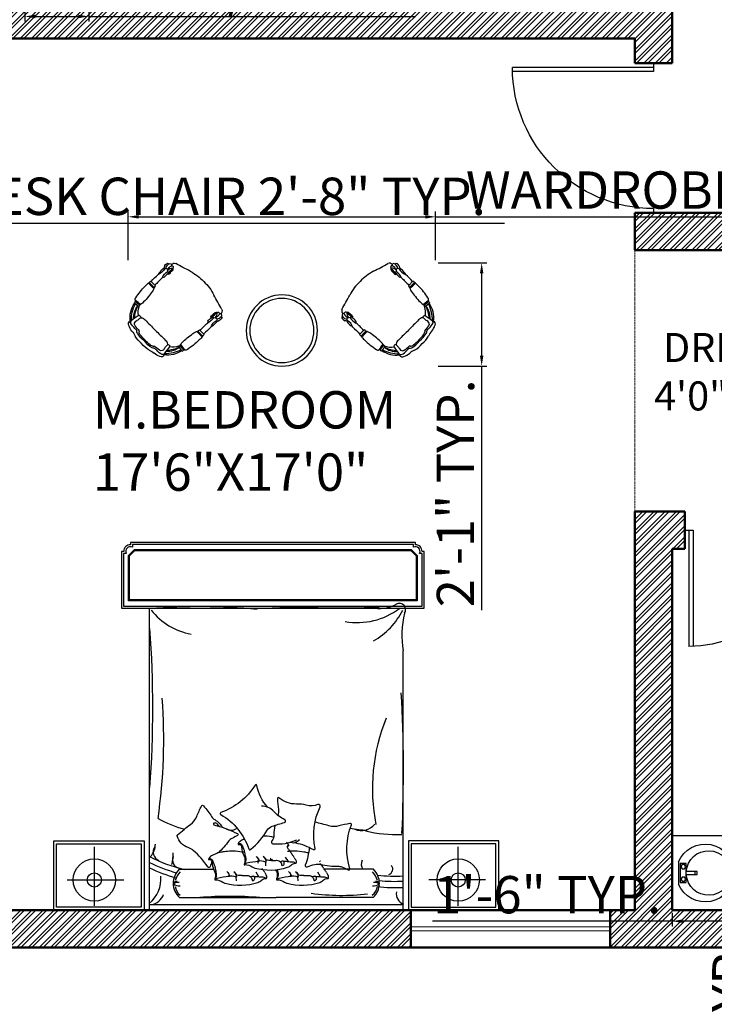
# Model space of a CAD drawing. Units: inches. Extents: x 3590 to 5167, y 65 to 1917.
# Tile 17 of 100: x 3716 to 3884, y 1312 to 1549. Entities that reach past the tile are written whole.
import ezdxf

# ---------------------------------------------------------------- set-up
doc = ezdxf.new("R2010")
doc.units = ezdxf.units.IN
doc.linetypes.add('DASHED', pattern=[0.75, 0.5, -0.25])
for name, color, linetype, lineweight in [('A-ANNO-DIMS', 2, 'Continuous', 18), ('A-AREA-IDEN', 7, 'Continuous', 18), ('A-DOOR', 3, 'Continuous', 25), ('A-FLOR-FIXT', 8, 'Continuous', 18), ('A-FURN', 21, 'Continuous', 18), ('A-GLAZ', 4, 'Continuous', 18), ('A-WALL', 7, 'Continuous', 50), ('A-WALL-PATT', 251, 'Continuous', 13), ('S-BEAM-OVHD', 7, 'DASHED', 18)]:
    doc.layers.add(name, color=color, linetype=linetype, lineweight=lineweight)
for name, color, linetype in [('FUR', 42, 'Continuous'), ('furn', 7, 'Continuous'), ('HA-FUR', 8, 'Continuous'), ('HA-P', 8, 'Continuous'), ('SAN', 5, 'Continuous'), ('SANTEH', 7, 'Continuous'), ('wood', 26, 'Continuous')]:
    doc.layers.add(name, color=color, linetype=linetype)
doc.styles.get("Standard").update_dxf_attribs({"font": 'arial.ttf'})
doc.dimstyles.new('ISO-25', dxfattribs={"dimtxt": 9, "dimasz": 2.5, "dimexe": 1.25, "dimexo": 0.625, "dimtad": 1, "dimdec": 1, "dimlunit": 3, "dimtxsty": 'Standard', "dimcen": 2.5, "dimadec": 0, "dimazin": 0, "dimtfac": 1, "dimtdec": 1, "dimtmove": 0, "dimatfit": 3, "dimfxl": 1, "dimarcsym": 0})

# ---------------------------------------------------------------- blocks, each defined once
blk = doc.blocks.new('D2')
for p, q in [((1, 0), (1, 28)), ((2, 0), (2, 27.98)), ((0, 0), (2, 0)), ((29, 0), (30, 0))]:
    blk.add_line(p, q)
at = {"ltscale": 0.5}
blk.add_arc((1, 0), 28, 0, 90, dxfattribs=at)
blk = doc.blocks.new('D1')
for p, q in [((1, 0), (1, 34)), ((2, 0), (2, 33.99)), ((0, 0), (2, 0)), ((35, 0), (36, 0))]:
    blk.add_line(p, q)
at = {"ltscale": 0.5}
blk.add_arc((1, 0), 34, 0, 90, dxfattribs=at)
blk = doc.blocks.new('r11')
at = {"layer": 'SANTEH', "ltscale": 5}
for p, q in [((0, 0), (600, 0)), ((0, -600), (0, 0)), ((600, 0), (600, -600)), ((210.5, -50), (389.5, -50)), ((210.5, -50), (210.5, -50)), ((223.8, -63.2), (376.2, -63.2)), ((223.8, -113.2), (223.8, -63.2)), ((232.7, -78.7), (249.2, -69.1)), ((232.7, -97.7), (232.7, -78.7)), ((249.2, -69.1), (265.7, -78.7)), ((265.7, -78.7), (265.7, -97.7)), ((334.3, -78.7), (350.8, -69.1)), ((334.3, -97.7), (334.3, -78.7)), ((350.8, -69.1), (367.3, -78.7)), ((367.3, -78.7), (367.3, -97.7)), ((376.2, -63.2), (376.2, -113.2)), ((376.2, -113.2), (223.8, -113.2)), ((249.2, -107.2), (232.7, -97.7)), ((265.7, -97.7), (249.2, -107.2)), ((288, -201.6), (288, -113.2)), ((312, -113.2), (312, -201.6)), ((350.8, -107.2), (334.3, -97.7)), ((367.3, -97.7), (350.8, -107.2)), ((312, -184.3), (288, -184.3)), ((312, -201.6), (288, -201.6)), ((600, -600), (0, -600))]:
    blk.add_line(p, q, dxfattribs=at)
for centre, radius, start, end in [((300, -266.2), 234, 112.50001, 67.49999), ((300, -293), 180.2, 93.8183, 86.1817)]:
    blk.add_arc(centre, radius, start, end, dxfattribs=at)
blk = doc.blocks.new('A$C0A42580C')
at = {"layer": 'SAN'}
for p, q in [((0.2873, 0.0301), (0.2873, 0.4484)), ((2.8678, 0.0301), (2.8678, 0.4484)), ((0.0949, 0.2135), (0.4958, 0.2135)), ((3.0601, 0.2135), (2.6592, 0.2135))]:
    blk.add_line(p, q, dxfattribs=at)
for centre, radius in [((0.2873, 0.2135), 0.15), ((2.8678, 0.2135), 0.15), ((0.2873, 0.2135), 0.05), ((2.8678, 0.2135), 0.05)]:
    blk.add_circle(centre, radius, dxfattribs=at)
at = {"layer": 'wood'}
for p, q in [((0.6775, 0.8851), (0.6775, 2.1392)), ((2.4775, 0.8016), (2.4775, 1.838)), ((2.4775, 0), (2.4775, 0.8016)), ((1.6633, 0.3438), (1.6434, 0.3761)), ((0.888, 0.289), (1.1327, 0.289)), ((1.5, 0.3423), (1.5016, 0.3142)), ((2.267, 0.289), (1.9163, 0.289)), ((1.2906, 0.2348), (1.2921, 0.2067)), ((1.4538, 0.2362), (1.434, 0.2685)), ((1.7287, 0.2348), (1.7302, 0.2067)), ((1.8919, 0.2362), (1.8721, 0.2685)), ((0.8909, 0.089), (1.5775, 0.089)), ((2.2642, 0.089), (1.5775, 0.089)), ((0.6775, 0.039), (2.4775, 0.039)), ((0.6775, 0), (2.4775, 0))]:
    blk.add_line(p, q, dxfattribs=at)
blk.add_lwpolyline([(0.6775, 0), (0.6775, 0.8851)], dxfattribs=at)
for points in [[(1.516, 0.7294, -0.128392), (1.4401, 0.8834, 0.70791), (1.427, 0.8863, -0.16964), (1.1848, 0.6919, 0.664036), (1.184, 0.6776, -0.184649), (1.3819, 0.4332, 0.662242), (1.3969, 0.4309, 0.078539), (1.5137, 0.5669, -0.1736), (1.5484, 0.5947, -0.02159), (1.6357, 0.6205, 0.697276), (1.6379, 0.6405, -0.093019), (1.5606, 0.699, 0.216632), (1.4719, 0.7371, -2.511293)], [(1.6795, 0.4818, 0.263265), (1.7191, 0.4839, -0.026108), (1.743, 0.4973, 0.027613), (1.7137, 0.4764, -0.089259), (1.8403, 0.429, 0.662242), (1.8528, 0.4376, -0.162037), (1.8882, 0.732, 0.676499), (1.8733, 0.748, -0.160513), (1.7901, 0.7439, 0.07473), (1.7202, 0.7523, -0.187721), (1.5966, 0.7963, 0.70791), (1.5851, 0.7895, -0.010003), (1.5921, 0.7143, -0.07079), (1.5891, 0.6719, 0.099539)], [(1.1211, 0.3454, 0.032543), (1.1095, 0.3091, -0.658965), (1.0917, 0.3063, 0.074753), (0.9887, 0.4234, 0.100988), (0.953, 0.4429, -0.270711), (0.8753, 0.5273, -0.276825), (0.8775, 0.5337, -0.014937), (0.9701, 0.6081, 0.134834), (1.0135, 0.6643, -0.023706), (1.0474, 0.7372, -0.664036), (1.0616, 0.7394, -0.035987), (1.119, 0.6627, 0.118631), (1.1415, 0.6412, -0.132738), (1.1955, 0.5864)], [(1.1759, 0.5928, 0.013884), (1.1549, 0.6131, 0.174178), (1.1437, 0.6177, 0.104076), (1.1358, 0.6165, 0.389829), (1.1324, 0.6097, 0.296089), (1.1415, 0.6019, -0.036701), (1.1572, 0.5985, -0.040547), (1.3022, 0.543, -0.70791), (1.3021, 0.5296, -0.016811), (1.2631, 0.5085, 0.11866), (1.2414, 0.4904, -0.048791), (1.1649, 0.4055, 0.103757)], [(1.5674, 0.601, 0.057807), (1.5606, 0.5339, -0.173425), (1.5457, 0.49, 0.589988), (1.5538, 0.4706, 0.137312), (1.7236, 0.4985, 0.137312)], [(1.8113, 0.4446, -0.069098), (1.7831, 0.3187, 0.658965), (1.7961, 0.3062, -0.049789), (1.8516, 0.3234, -0.103757), (1.8905, 0.3233, 0.055725), (2.0203, 0.3103, -0.11866), (2.0478, 0.304, 0.016811), (2.0881, 0.2856, 0.70791), (2.0989, 0.2936, -0.16964), (2.1104, 0.604, 0.664036), (2.1001, 0.6139, 0.023706), (2.0214, 0.597, -0.134834), (1.9505, 0.5976, 0.012748), (1.8522, 0.6228)], [(1.3107, 0.4764, 0.145733), (1.3069, 0.4677, 0.488583), (1.3089, 0.4657, -0.012138), (1.3131, 0.4661, -0.125673), (1.3213, 0.4646, -0.750706)], [(1.3153, 0.4751, -0.274893), (1.3379, 0.4529, 0.051436), (1.3468, 0.4293, -0.086628), (1.3532, 0.4078, 0.040196), (1.3593, 0.3772, -0.184744), (1.3556, 0.3344, -2.554464)], [(1.317, 0.4683, -0.060098), (1.3283, 0.4571, -0.16247), (1.3313, 0.4487, 0.120018), (1.3493, 0.3815, -0.060072), (1.3541, 0.3695, -0.13107), (1.3541, 0.3395, -0.024415), (1.3534, 0.3373, 0.070398), (1.3503, 0.3233, 0.528689), (1.3524, 0.3216, -0.069388), (1.3557, 0.3222, -0.158233), (1.4075, 0.3065, 0.085461), (1.4255, 0.2981, 0.147196), (1.6571, 0.3041, 0.10985), (1.6823, 0.3191, -0.179095), (1.7126, 0.3319, -2.318897)], [(1.1013, 0.3688, 0.145733), (1.0975, 0.3601, 0.488583), (1.0995, 0.3581, -0.012138), (1.1036, 0.3585, -0.125673), (1.1119, 0.357, -0.750706)], [(1.1059, 0.3675, -0.274893), (1.1285, 0.3453, 0.051436), (1.1373, 0.3217, -0.086628), (1.1438, 0.3003, 0.040196), (1.1499, 0.2696, -0.184744), (1.1462, 0.2269, -2.554464)], [(1.1076, 0.3607, -0.060098), (1.1189, 0.3495, -0.16247), (1.1219, 0.3411, 0.120018), (1.1399, 0.2739, -0.060072), (1.1447, 0.2619, -0.13107), (1.1447, 0.2319, -0.024415), (1.144, 0.2297, 0.070398), (1.1409, 0.2157, 0.528689), (1.143, 0.2141, -0.069388), (1.1463, 0.2146, -0.158233), (1.1981, 0.1989, 0.085461), (1.2161, 0.1905, 0.147196), (1.4477, 0.1965, 0.10985), (1.4728, 0.2115, -0.179095), (1.5032, 0.2244, -2.318897)], [(1.4359, 0.3803, -0.198519), (1.452, 0.3494, 0.826402), (1.4558, 0.349, 0.095956), (1.4561, 0.3528, 0.242899), (1.4461, 0.3686, -17.523452)], [(1.5447, 0.3525, -0.083557), (1.507, 0.3546, 0.203162), (1.4851, 0.3792, -0.208037), (1.5043, 0.3409, 0.124669), (1.4432, 0.3469, 0.965934)], [(1.5394, 0.3688, 0.145733), (1.5356, 0.3601, 0.488583), (1.5376, 0.3581, -0.012138), (1.5418, 0.3585, -0.125673), (1.55, 0.357, -0.750706)], [(1.5447, 0.3525, -0.008229), (1.5728, 0.3519, 0.033691)], [(1.5728, 0.3519, -0.46905), (1.6152, 0.321, 0.420988), (1.62, 0.3169, 0.857652), (1.6221, 0.3484, 0.548526)], [(1.3509, 0.3219, -0.117141), (1.3688, 0.335, -0.025084), (1.4533, 0.348, 0.033691)], [(1.5721, 0.286, 0.022869), (1.578, 0.2739, -0.060072), (1.5828, 0.2619, -0.13107), (1.5828, 0.2319, -0.024415), (1.5821, 0.2297, 0.070398), (1.579, 0.2157, 0.528689), (1.5811, 0.2141, -0.069388), (1.5844, 0.2146, -0.158233), (1.6362, 0.1989, 0.085461), (1.6542, 0.1905, 0.147196), (1.8858, 0.1965, 0.10985), (1.911, 0.2115, -0.179095), (1.9413, 0.2244, -2.318897)], [(1.5838, 0.2873, 0.023398), (1.588, 0.2696, -0.184744), (1.5843, 0.2269, -2.554464)], [(1.603, 0.3451, -0.099719), (1.6221, 0.3484, 0.102691)], [(1.6214, 0.3487, -0.010168), (1.6558, 0.3447, 0.033691), (1.6907, 0.3423, -0.220869), (1.7148, 0.3311, -0.288972)], [(1.1415, 0.2143, -0.117141), (1.1594, 0.2274, -0.025084), (1.2439, 0.2405, 0.033691)], [(1.2265, 0.2728, -0.198519), (1.2426, 0.2418, 0.826402), (1.2463, 0.2415, 0.095956), (1.2467, 0.2452, 0.242899), (1.2366, 0.2611, -17.523452)], [(1.3353, 0.2449, -0.083557), (1.2976, 0.247, 0.203162), (1.2757, 0.2717, -0.208037), (1.2948, 0.2333, 0.124669), (1.2338, 0.2393, 0.965934)], [(1.3353, 0.2449, -0.008229), (1.3633, 0.2443, 0.033691)], [(1.3633, 0.2443, -0.46905), (1.4058, 0.2134, 0.420988), (1.4106, 0.2093, 0.857652), (1.4127, 0.2408, 0.548526)], [(1.3936, 0.2375, -0.099719), (1.4127, 0.2408, 0.102691)], [(1.412, 0.2411, -0.010168), (1.4464, 0.2371, 0.033691), (1.4812, 0.2348, -0.220869), (1.5054, 0.2235, -0.288972)], [(1.5796, 0.2143, -0.117141), (1.5975, 0.2274, -0.025084), (1.682, 0.2405, 0.033691)], [(1.6646, 0.2728, -0.198519), (1.6807, 0.2418, 0.826402), (1.6845, 0.2415, 0.095956), (1.6848, 0.2452, 0.242899), (1.6748, 0.2611, -17.523452)], [(1.7734, 0.2449, -0.083557), (1.7357, 0.247, 0.203162), (1.7138, 0.2717, -0.208037), (1.733, 0.2333, 0.124669), (1.6719, 0.2393, 0.965934)], [(1.7734, 0.2449, -0.008229), (1.8015, 0.2443, 0.033691)], [(1.8015, 0.2443, -0.46905), (1.8439, 0.2134, 0.420988), (1.8487, 0.2093, 0.857652), (1.8508, 0.2408, 0.548526)], [(1.8317, 0.2375, -0.099719), (1.8508, 0.2408, 0.102691)], [(1.8501, 0.2411, -0.010168), (1.8845, 0.2371, 0.033691), (1.9193, 0.2348, -0.220869), (1.9435, 0.2235, -0.288972)]]:
    blk.add_lwpolyline(points, format="xyb", dxfattribs=at)
for points in [[(0.64, 0), (0, 0), (0, 0.49), (0.64, 0.49)], [(2.515, 0), (3.155, 0), (3.155, 0.49), (2.515, 0.49)], [(0.62, 0.02), (0.02, 0.02), (0.02, 0.47), (0.62, 0.47)], [(2.535, 0.02), (3.135, 0.02), (3.135, 0.47), (2.535, 0.47)]]:
    blk.add_lwpolyline(points, close=True, dxfattribs=at)
for centre, radius, start, end in [((2.3125, 2.3833), 0.2443, 254.1515, 300.95574), ((2.4501, 2.1309), 0.0445, 324.18954, 118.92203), ((1.0344, -2.14), 4.292, 84.56078, 94.7164), ((1.0494, 2.4026), 0.4515, 217.47941, 260.35986), ((2.0208, -11.0786), 13.2288, 88.75549, 92.51133), ((2.1491, 2.5471), 0.5083, 260.65485, 306.44155), ((2.0168, 2.3573), 0.5127, 299.08175, 333.44367), ((3.1371, 1.9502), 0.669, 166.6404, 189.65708), ((-7.0839, 1.4328), 7.7858, 355.84817, 4.15183), ((-7.2439, 0.9937), 9.7233, 357.34474, 3.23068), ((-3.167, 1.2143), 3.9465, 351.77286, 4.18386), ((3.5803, 0.8622), 1.3213, 157.81295, 191.15154), ((1.1611, 1.4181), 0.8768, 241.21362, 254.41879), ((1.2583, 0.6364), 0.0695, 238.58923, 301.92671), ((1.7861, -2.1601), 2.7557, 80.89877, 83.46656), ((2.181, 0.6859), 0.1221, 247.37754, 321.13165), ((2.4192, 1.3819), 0.8461, 255.77539, 273.25587), ((1.3546, 0.4469), 0.0529, 114.21284, 146.15395), ((2.6126, -2.3504), 3.1201, 113.83178, 114.21284), ((1.4714, 0.0722), 0.4528, 80.62397, 88.74059), ((1.4035, -0.3388), 0.8693, 79.71489, 80.62397), ((0.5904, 0.4689), 0.13, 317.38218, 359.70393), ((0.7723, 0.4131), 0.0674, 147.68233, 245.79865), ((1.6301, 0.4539), 0.0342, 31.14095, 54.95422), ((1.6709, 0.4489), 0.0156, 131.9623, 212.08127), ((1.6729, 0.4422), 0.0178, 140.41793, 157.63267), ((1.7235, 0.4818), 0.0777, 212.08127, 227.364), ((1.6635, 0.4499), 0.00568, 95.52245, 140.41793), ((1.5664, 0.4154), 0.1086, 24.20989, 31.14095), ((1.6627, 0.4587), 0.00309, 275.52245, 24.20989), ((1.6391, 0.3902), 0.0469, 17.32618, 47.364), ((1.1611, 1.3191), 1.0568, 242.76671, 257.10398), ((0.0312, 0.4583), 0.8174, 350.42368, 356.2506), ((0.9021, 0.3562), 0.0605, 155.8342, 254.41058), ((1.1452, 0.3394), 0.0529, 114.21284, 146.15395), ((2.4032, -2.458), 3.1201, 113.55686, 114.21284), ((1.2046, 0.2912), 0.121, 99.42032, 113.55686), ((1.2774, -0.1478), 0.5659, 95.90379, 99.42032), ((1.2626, -0.005), 0.4223, 88.74059, 95.90379), ((1.2619, -0.0354), 0.4528, 80.62397, 88.74059), ((1.1941, -0.4464), 0.8693, 79.45871, 80.62397), ((1.4207, 0.3463), 0.0342, 31.14095, 54.95422), ((1.4614, 0.3413), 0.0156, 131.9623, 212.08127), ((1.357, 0.3078), 0.1086, 24.20989, 31.14095), ((1.4533, 0.3511), 0.00309, 275.52245, 24.20989), ((1.7007, -0.005), 0.4223, 88.74059, 95.90379), ((1.7106, 0.4125), 0.028, 197.32618, 226.17302), ((1.6431, 0.3422), 0.0695, 26.61764, 46.17302), ((1.8202, 0.431), 0.1287, 206.61764, 215.96192), ((1.7001, -0.0354), 0.4528, 80.62397, 88.74059), ((1.6975, 0.3419), 0.023, 350.76434, 35.96192), ((1.6322, -0.4464), 0.8693, 78.43923, 80.62397), ((2.2511, 0.3256), 0.071, 155.86842, 211.04513), ((1.1611, 1.3191), 1.0937, 243.75553, 254.4906), ((1.1611, 1.2816), 1.0937, 243.75553, 254.38927), ((0.9846, 0.1903), 0.1381, 134.39284, 227.23745), ((1.4635, 0.3347), 0.0178, 140.41793, 157.63267), ((1.4541, 0.3424), 0.00568, 95.52245, 140.41793), ((1.5012, 0.305), 0.028, 197.32618, 226.17302), ((1.4337, 0.2347), 0.0695, 26.61764, 46.17302), ((1.715, 0.3349), 0.00379, 207.1817, 328.02977), ((1.7058, 0.3406), 0.0145, 328.02977, 350.76434), ((1.9016, 0.3347), 0.0178, 140.41793, 157.63267), ((1.9522, 0.3743), 0.0777, 212.08127, 227.364), ((1.8922, 0.3424), 0.00568, 95.52245, 140.41793), ((1.8678, 0.2827), 0.0469, 17.32618, 47.364), ((1.9393, 0.305), 0.028, 197.32618, 226.17302), ((1.8718, 0.2347), 0.0695, 26.61764, 46.17302), ((2.1704, 0.1903), 0.1381, 312.76255, 45.60716), ((2.3616, 0.2915), 0.0419, 290.78583, 35.36309), ((0.5293, 0.2241), 0.2307, 309.63048, 4.27465), ((0.9986, 0.1735), 0.1427, 136.58239, 164.9725), ((1.6108, 0.3235), 0.1287, 206.61764, 215.96192), ((1.5055, 0.2273), 0.00379, 207.1817, 328.02977), ((1.4881, 0.2344), 0.023, 350.76434, 35.96192), ((1.4964, 0.233), 0.0145, 328.02977, 350.76434), ((2.0489, 0.3235), 0.1287, 206.61764, 215.96192), ((1.9436, 0.2273), 0.00379, 207.1817, 328.02977), ((1.9262, 0.2344), 0.023, 350.76434, 35.96192), ((1.9345, 0.233), 0.0145, 328.02977, 350.76434), ((2.1565, 0.1735), 0.1427, 15.0275, 43.41761), ((2.4192, 1.2667), 1.0261, 263.09035, 273.25587), ((2.4192, 1.2667), 1.0629, 263.94374, 273.25587), ((0.8396, 0.185), 0.0112, 314.89662, 45.10338), ((0.8413, 0.1846), 0.0128, 299.47062, 57.44416), ((0.8844, 0.2286), 0.0569, 229.70587, 281.11527), ((0.8802, 0.1371), 0.0592, 81.47786, 123.11925), ((0.8698, 0.1793), 0.0229, 77.14902, 159.1786), ((0.9466, 0.1765), 0.0862, 185.53723, 234.68694), ((2.2085, 0.1765), 0.0862, 305.31306, 354.46277), ((2.2706, 0.2286), 0.0569, 258.88473, 310.29413), ((2.2749, 0.1371), 0.0592, 56.88075, 98.52214), ((2.2853, 0.1793), 0.0229, 20.8214, 102.85098), ((2.4192, 1.2218), 1.0629, 263.23622, 273.25587), ((2.3138, 0.1846), 0.0128, 122.55584, 240.52938), ((2.3154, 0.185), 0.0112, 134.89662, 225.10338), ((0.6729, 0.151), 0.1135, 279.23824, 338.73819), ((1.2481, -2.5919), 2.6893, 85.4722, 94.5278), ((2.0447, 1.7022), 1.5979, 262.13639, 276.48786), ((2.508, 0.1152), 0.0792, 169.94668, 248.24015)]:
    blk.add_arc(centre, radius, start, end, dxfattribs=at)
blk = doc.blocks.new('A$C623F1DA0')
at = {"layer": 'FUR'}
blk.add_lwpolyline([(0.628, 2.912, 0.414214), (0.562, 2.978), (0.562, 3), (0, 3), (0, 0), (0.562, 0), (0.562, 0.022, 0.414214), (0.628, 0.088), (0.65, 0.088), (0.65, 2.912)], format="xyb", close=True, dxfattribs=at)
at = {"layer": 'HA-FUR'}
blk.add_lwpolyline([(0.6034, 2.892, 0.710288), (0.542, 2.9534), (0.542, 2.98), (0.02, 2.98), (0.02, 0.02), (0.542, 0.02), (0.542, 0.0466, 0.710288), (0.6034, 0.108), (0.63, 0.108), (0.63, 2.892)], format="xyb", close=True, dxfattribs=at)
at = {"layer": 'HA-P'}
for points in [[(0.07, 2.93), (0.5213, 2.93), (0.58, 2.8713), (0.58, 0.1287), (0.5213, 0.07), (0.07, 0.07)], [(0.08, 2.92), (0.5171, 2.92), (0.57, 2.8671), (0.57, 0.1329), (0.5171, 0.08), (0.08, 0.08)]]:
    blk.add_lwpolyline(points, close=True, dxfattribs=at)
blk = doc.blocks.new('CHAIR6')
at = {"layer": 'furn'}
for p, q in [((0.41, 0.26), (0.4094, 0.3185)), ((0.4281, 0.3181), (0.4272, 0.263)), ((0.41, -0.26), (0.4094, -0.3185)), ((0.4281, -0.3181), (0.4272, -0.263))]:
    blk.add_line(p, q, dxfattribs=at)
for centre in [(0.2174, 0.2867), (0.2187, 0.2766), (0.22, 0.2683), (0.2209, 0.2599), (0.2221, 0.2517), (0.4052, 0.3065), (0.4053, 0.3148), (0.4053, 0.2897), (0.4054, 0.2981), (0.4054, 0.2729), (0.4055, 0.2812), (0.4056, 0.2643), (0.2231, 0.2433), (0.2221, -0.2517), (0.2231, -0.2433), (0.2174, -0.2867), (0.2187, -0.2766), (0.22, -0.2683), (0.2209, -0.2599), (0.4052, -0.3065), (0.4053, -0.2897), (0.4053, -0.3148), (0.4054, -0.2981), (0.4054, -0.2729), (0.4055, -0.2812), (0.4056, -0.2643)]:
    blk.add_circle(centre, 0.00425, dxfattribs=at)
for centre, radius, start, end in [((0.2315, 0.0781), 0.2058, 99.53594, 142.96968), ((0.288, -0.009), 0.2959, 107.467, 135.69066), ((0.1998, 0.3299), 0.0425, 267.37882, 299.53851), ((0.5076, 0.3087), 0.3105, 183.92135, 193.66405), ((0.91, 0.35), 0.6998, 184.95819, 189.17441), ((0.2369, 0.2913), 0.0162, 83.97727, 174.0092), ((2.2364, 0.5463), 2.0315, 187.16408, 188.67417), ((0.3719, -0.3167), 0.6382, 90.6066, 102.05541), ((0.3772, 0.1685), 0.1534, 77.89638, 94.52684), ((0.357, 0.3514), 0.1057, 274.42127, 300.14813), ((3.3638, 0.3149), 2.9628, 179.90105, 181.14792), ((0.4178, 0.2794), 0.04, 75.21702, 102.18253), ((0.4118, 0.3013), 0.0413, 267.60688, 291.9537), ((0.4709, 1.0442), 0.7753, 266.77935, 273.30843), ((0.4807, -0.3094), 0.6241, 87.1388, 94.84242), ((0.5163, 0.348), 0.0344, 262.5365, 295.12391), ((0.5543, 0.4048), 0.1004, 244.96152, 286.92621), ((0.5583, 0.1491), 0.1284, 78.32163, 109.43704), ((0.5171, 0.2599), 0.0105, 7.92951, 98.404), ((0.5475, 0.4175), 0.1574, 262.69111, 279.4279), ((0.5573, 0.1986), 0.1211, 80.56871, 102.58021), ((0.5763, 0.2592), 0.00554, 151.0446, 320.63906), ((0.5726, 0.2536), 0.00119, 58.88827, 217.83169), ((0.5864, 0.2986), 0.0481, 252.15364, 277.04405), ((0.5749, 0.272), 0.00992, 261.06044, 17.03518), ((0.569, 0.3057), 0.0148, 11.93121, 56.71364), ((0.6, 0.6108), 0.3491, 266.32513, 275.76594), ((0.5857, 0.2587), 0.00592, 143.235, 315.8485), ((0.5574, 0.3682), 0.0592, 293.70731, 312.31146), ((0.5811, 0.2921), 0.0168, 1.95853, 81.75781), ((0.5706, 0.2994), 0.0282, 299.26311, 346.05528), ((0.54, 0.2614), 0.0504, 352.19447, 0.49312), ((0.5958, 0.265), 0.012, 240.91565, 292.3604), ((0.5993, 0.2232), 0.0286, 84.23587, 104.22566), ((0.6205, 0.2416), 0.0492, 62.08685, 124.06689), ((0.5958, 0.2324), 0.05, 38.36456, 93.27362), ((0.6272, 0.2528), 0.0606, 83.33143, 123.59051), ((0.6147, 0.2731), 0.0542, 72.72663, 108.72189), ((0.6298, 0.2592), 0.03, 175.25421, 190.14236), ((0.6039, 0.2608), 0.00773, 242.68072, 299.22641), ((0.6055, 0.322), 0.0704, 267.27867, 279.33441), ((0.6233, 0.2599), 0.0167, 173.50236, 200.39748), ((0.6103, 0.2582), 0.0049, 236.84733, 330.71615), ((0.6462, 0.2619), 0.0322, 179.91617, 191.03659), ((0.6177, 0.2574), 0.00347, 207.27606, 12.12043), ((0.6201, 0.2638), 0.0117, 254.38571, 324.07897), ((0.7103, 0.267), 0.0896, 182.99093, 185.70819), ((0.6264, 0.2651), 0.00881, 232.86154, 349.28828), ((0.6287, 0.3179), 0.00734, 318.72654, 73.20464), ((0.6327, 0.2954), 0.0177, 352.68742, 85.29917), ((0.6348, 0.276), 0.0126, 270.96281, 46.15927), ((0.6241, 0.3083), 0.0303, 309.85115, 329.87174), ((0.651, 0.2582), 0.0349, 27.02079, 91.1191), ((5.5909, 1.6415), 5.0957, 195.56602, 197.11239), ((0.1754, 0.1139), 0.1594, 153.58586, 173.67646), ((0.0568, 0.1796), 0.0247, 65.10842, 167.8729), ((0.2078, 0.1391), 0.1575, 161.79448, 183.48135), ((0.076, 0.1763), 0.0215, 90.49656, 146.04111), ((0.0747, 0.2065), 0.00875, 210.7256, 277.12246), ((0.0962, 0.1341), 0.0336, 65.79003, 135.37187), ((1.2944, 7.3493), 7.2545, 260.32992, 260.96162), ((0.2204, 0.0839), 0.1637, 95.98601, 137.80844), ((0.2974, -0.0268), 0.2892, 108.96584, 130.74832), ((0.2701, 0.1022), 0.1479, 115.74239, 145.5422), ((0.1013, 0.1754), 0.0542, 340.13538, 9.97368), ((0.217, 0.2087), 0.0298, 85.88245, 112.38941), ((0.2036, 0.356), 0.1186, 277.54736, 281.93488), ((0.2433, 0.2647), 0.029, 238.53775, 274.93529), ((0.2506, 0.8795), 0.6438, 269.57373, 280.24813), ((0.2403, 0.0222), 0.2414, 165.22851, 185.28449), ((-0.0992, 0.1308), 0.1161, 336.07618, 0.28835), ((0.2703, 0.0325), 0.2394, 166.65717, 187.80685), ((0.064, 0.0801), 0.0277, 124.74206, 163.83274), ((0.0904, 0.0544), 0.0465, 139.20017, 173.50108), ((0.0085, 0.1198), 0.0432, 336.84052, 13.12552), ((0.0425, 0.1014), 0.0209, 307.26707, 6.28043), ((0.2344, 0.1031), 0.1711, 161.37859, 179.7853), ((0.1315, 0.2333), 0.0718, 252.51235, 277.4747), ((0.1416, 0.1481), 0.0139, 39.59763, 92.78598), ((0.1123, 0.1263), 0.0505, 352.81567, 37.47081), ((-4.0332, 0.095), 4.1956, 358.70239, 0.34145), ((0.3444, 0.019), 0.396, 357.24911, 18.10814), ((0.4579, 0.0143), 0.4162, 173.74932, 181.97518), ((0.2403, -0.0222), 0.2414, 174.71551, 194.77149), ((0.2703, -0.0325), 0.2394, 172.19315, 193.34283), ((0.4579, -0.0143), 0.4162, 178.02482, 186.25068), ((0.0904, -0.0544), 0.0465, 186.49892, 220.79983), ((-4.0332, -0.095), 4.1956, 359.65855, 1.29761), ((0.3444, -0.019), 0.396, 341.89186, 2.75089), ((-0.0992, -0.1308), 0.1161, 359.71165, 23.92382), ((0.1754, -0.1139), 0.1594, 186.32354, 206.41414), ((0.064, -0.0801), 0.0277, 196.16726, 235.25794), ((0.0085, -0.1198), 0.0432, 346.87448, 23.15948), ((0.2078, -0.1391), 0.1575, 176.51865, 198.20552), ((0.0425, -0.1014), 0.0209, 353.71957, 52.73293), ((0.2344, -0.1031), 0.1711, 180.2147, 198.62141), ((0.0962, -0.1341), 0.0336, 224.62813, 294.20997), ((0.1315, -0.2333), 0.0718, 82.5253, 107.48765), ((0.1416, -0.1481), 0.0139, 267.21402, 320.40237), ((0.1123, -0.1263), 0.0505, 322.52919, 7.18433), ((0.1013, -0.1754), 0.0542, 350.02632, 19.86462), ((5.5909, -1.6415), 5.0957, 162.88761, 164.43398), ((0.0568, -0.1796), 0.0247, 192.1271, 294.89158), ((0.076, -0.1763), 0.0215, 213.95889, 269.50344), ((0.0747, -0.2065), 0.00875, 82.87754, 149.2744), ((0.2315, -0.0781), 0.2058, 217.03032, 260.46406), ((1.2944, -7.3493), 7.2545, 99.03838, 99.67008), ((0.288, 0.009), 0.2959, 224.30934, 252.533), ((0.2204, -0.0839), 0.1637, 222.19156, 264.01399), ((0.2974, 0.0268), 0.2892, 229.25168, 251.03416), ((0.2701, -0.1022), 0.1479, 214.4578, 244.25761), ((0.5076, -0.3087), 0.3105, 166.33595, 176.07865), ((0.217, -0.2087), 0.0298, 247.61059, 274.11755), ((0.91, -0.35), 0.6998, 170.82559, 175.04181), ((0.2036, -0.356), 0.1186, 78.06512, 82.45264), ((2.2364, -0.5463), 2.0315, 171.32583, 172.83592), ((0.2433, -0.2647), 0.029, 85.06471, 121.46225), ((0.2506, -0.8795), 0.6438, 79.75187, 90.42627), ((0.357, -0.3514), 0.1057, 59.85187, 85.57873), ((0.1998, -0.3299), 0.0425, 60.46149, 92.62118), ((0.2369, -0.2913), 0.0162, 185.9908, 276.02273), ((0.3719, 0.3167), 0.6382, 257.94459, 269.3934), ((0.3772, -0.1685), 0.1534, 265.47316, 282.10362), ((3.3638, -0.3149), 2.9628, 178.85208, 180.09895), ((0.4178, -0.2794), 0.04, 257.81747, 284.78298), ((0.4118, -0.3013), 0.0413, 68.0463, 92.39312), ((0.4709, -1.0442), 0.7753, 86.69157, 93.22065), ((0.4807, 0.3094), 0.6241, 265.15758, 272.8612), ((0.5543, -0.4048), 0.1004, 73.07379, 115.03848), ((0.5163, -0.348), 0.0344, 64.87609, 97.4635), ((0.5171, -0.2599), 0.0105, 261.596, 352.07049), ((0.5583, -0.1491), 0.1284, 250.56296, 281.67837), ((0.5475, -0.4175), 0.1574, 80.5721, 97.30889), ((0.5573, -0.1986), 0.1211, 257.41979, 279.43129), ((0.5763, -0.2592), 0.00554, 39.36094, 208.9554), ((0.5726, -0.2536), 0.00119, 142.16831, 301.11173), ((0.5864, -0.2986), 0.0481, 82.95595, 107.84636), ((0.5749, -0.272), 0.00992, 342.96482, 98.93956), ((0.569, -0.3057), 0.0148, 303.28636, 348.06879), ((0.6, -0.6108), 0.3491, 84.23406, 93.67487), ((0.5857, -0.2587), 0.00592, 44.1515, 216.765), ((0.5574, -0.3682), 0.0592, 47.68854, 66.29269), ((0.5811, -0.2921), 0.0168, 278.24219, 358.04147), ((0.5706, -0.2994), 0.0282, 13.94472, 60.73689), ((0.5958, -0.265), 0.012, 67.6396, 119.08435), ((0.54, -0.2614), 0.0504, 359.50688, 7.80553), ((0.5993, -0.2232), 0.0286, 255.77434, 275.76413), ((0.5958, -0.2324), 0.05, 266.72638, 321.63544), ((0.6205, -0.2416), 0.0492, 235.93311, 297.91315), ((0.6272, -0.2528), 0.0606, 236.40949, 276.66857), ((0.6147, -0.2731), 0.0542, 251.27811, 287.27337), ((0.6298, -0.2592), 0.03, 169.85764, 184.74579), ((0.6039, -0.2608), 0.00773, 60.77359, 117.31928), ((0.6055, -0.322), 0.0704, 80.66559, 92.72133), ((0.6233, -0.2599), 0.0167, 159.60252, 186.49764), ((0.6103, -0.2582), 0.0049, 29.28385, 123.15267), ((0.6462, -0.2619), 0.0322, 168.96341, 180.08383), ((0.6177, -0.2574), 0.00347, 347.87957, 152.72394), ((0.6201, -0.2638), 0.0117, 35.92103, 105.61429), ((0.7103, -0.267), 0.0896, 174.29181, 177.00907), ((0.6264, -0.2651), 0.00881, 10.71172, 127.13846), ((0.6287, -0.3179), 0.00734, 286.79536, 41.27346), ((0.6327, -0.2954), 0.0177, 274.70083, 7.31258), ((0.6348, -0.276), 0.0126, 313.84073, 89.03719), ((0.6241, -0.3083), 0.0303, 30.12826, 50.14885), ((0.651, -0.2582), 0.0349, 268.8809, 332.97921)]:
    blk.add_arc(centre, radius, start, end, dxfattribs=at)
blk = doc.blocks.new('A$C78847651')
at = {"layer": 'furn'}
for radius in [0.3, 0.27]:
    blk.add_circle((1.2923, 0.5659), radius, dxfattribs=at)
at = {"layer": 'furn', "rotation": 315}
blk.add_blockref('CHAIR6', (0.1103, 0.6765), dxfattribs=at)
at = {"layer": 'furn', "xscale": -1, "rotation": 44.99999999999991}
blk.add_blockref('CHAIR6', (2.4743, 0.6765), dxfattribs=at)
blk = doc.blocks.new('*D290')
at = {"layer": 'A-ANNO-DIMS', "color": 0, "lineweight": -2, "transparency": 16777216}
for p, q in [((3742.44, 1491.53), (3742.44, 1503.26)), ((3744.94, 1502.01), (3813.99, 1502.01)), ((3816.49, 1491.53), (3816.49, 1503.26)), ((3816.49, 1502.01), (3953, 1502.01))]:
    blk.add_line(p, q, dxfattribs=at)
at = {"layer": 'A-ANNO-DIMS', "color": 0, "transparency": 16777216}
for points in [[(3744.94, 1502.43), (3744.94, 1501.59), (3742.44, 1502.01)], [(3813.99, 1502.43), (3813.99, 1501.59), (3816.49, 1502.01)]]:
    blk.add_solid(points, dxfattribs=at)
at = {"layer": 'Defpoints', "color": 0, "transparency": 16777216}
for p in [(3816.49, 1502.01), (3742.44, 1490.9), (3816.49, 1490.9)]:
    blk.add_point(p, dxfattribs=at)
at = {"layer": 'A-ANNO-DIMS', "color": 0, "transparency": 16777216, "insert": (3885.99, 1507.29), "char_height": 9, "attachment_point": 5}
blk.add_mtext('WARDROBE 6\'-2" TYP.', dxfattribs=at)
blk = doc.blocks.new('*D291')
at = {"layer": 'A-ANNO-DIMS', "color": 0, "lineweight": -2, "transparency": 16777216}
for p, q in [((3817.11, 1490.9), (3828.84, 1490.9)), ((3827.59, 1488.4), (3827.59, 1468.54)), ((3817.11, 1466.04), (3828.84, 1466.04)), ((3827.59, 1466.04), (3827.59, 1407.27))]:
    blk.add_line(p, q, dxfattribs=at)
at = {"layer": 'A-ANNO-DIMS', "color": 0, "transparency": 16777216}
for points in [[(3827.18, 1488.4), (3828.01, 1488.4), (3827.59, 1490.9)], [(3827.18, 1468.54), (3828.01, 1468.54), (3827.59, 1466.04)]]:
    blk.add_solid(points, dxfattribs=at)
at = {"layer": 'Defpoints', "color": 0, "transparency": 16777216}
for p in [(3816.49, 1490.9), (3816.49, 1466.04), (3827.59, 1466.04)]:
    blk.add_point(p, dxfattribs=at)
at = {"layer": 'A-ANNO-DIMS', "color": 0, "transparency": 16777216, "insert": (3822.45, 1435.4), "char_height": 9, "attachment_point": 5, "rotation": 90}
blk.add_mtext('2\'-1" TYP.', dxfattribs=at)
blk = doc.blocks.new('*D302')
at = {"layer": 'A-ANNO-DIMS', "color": 0, "lineweight": -2, "transparency": 16777216}
for p, q in [((3662.49, 1504.69), (3662.49, 1499.25)), ((3694.59, 1504.69), (3694.59, 1499.25)), ((3664.99, 1500.5), (3692.09, 1500.5)), ((3694.59, 1500.5), (3833.1, 1500.5))]:
    blk.add_line(p, q, dxfattribs=at)
at = {"layer": 'A-ANNO-DIMS', "color": 0, "transparency": 16777216}
for points in [[(3664.99, 1500.91), (3664.99, 1500.08), (3662.49, 1500.5)], [(3692.09, 1500.91), (3692.09, 1500.08), (3694.59, 1500.5)]]:
    blk.add_solid(points, dxfattribs=at)
at = {"layer": 'Defpoints', "color": 0, "transparency": 16777216}
for p in [(3662.49, 1505.31), (3694.59, 1505.31), (3694.59, 1500.5)]:
    blk.add_point(p, dxfattribs=at)
at = {"layer": 'A-ANNO-DIMS', "color": 0, "transparency": 16777216, "insert": (3765.1, 1505.78), "char_height": 9, "attachment_point": 5}
blk.add_mtext('DESK CHAIR 2\'-8" TYP.', dxfattribs=at)
blk = doc.blocks.new('*D305')
at = {"layer": 'A-ANNO-DIMS', "color": 0, "lineweight": -2, "transparency": 16777216}
for p, q in [((3717.55, 1553.37), (3717.55, 1549.03)), ((3732.94, 1553.37), (3732.94, 1549.03)), ((3720.05, 1550.28), (3730.44, 1550.28)), ((3732.94, 1550.28), (3811.67, 1550.28))]:
    blk.add_line(p, q, dxfattribs=at)
at = {"layer": 'A-ANNO-DIMS', "color": 0, "transparency": 16777216}
for points in [[(3720.05, 1550.7), (3720.05, 1549.86), (3717.55, 1550.28)], [(3730.44, 1550.7), (3730.44, 1549.86), (3732.94, 1550.28)]]:
    blk.add_solid(points, dxfattribs=at)
at = {"layer": 'Defpoints', "color": 0, "transparency": 16777216}
for p in [(3717.55, 1554), (3732.94, 1554), (3732.94, 1550.28)]:
    blk.add_point(p, dxfattribs=at)
at = {"layer": 'A-ANNO-DIMS', "color": 0, "transparency": 16777216, "insert": (3773.56, 1555.56), "char_height": 9, "attachment_point": 5}
blk.add_mtext('1\'-3 1/2" TYP.', dxfattribs=at)
blk = doc.blocks.new('*D306')
at = {"layer": 'A-ANNO-DIMS', "color": 0, "lineweight": -2, "transparency": 16777216}
for p, q in [((3892, 1352.87), (3895.31, 1352.87)), ((3894.06, 1350.37), (3894.06, 1337.5)), ((3892, 1335), (3895.31, 1335)), ((3894.06, 1335), (3894.06, 1193.58))]:
    blk.add_line(p, q, dxfattribs=at)
at = {"layer": 'A-ANNO-DIMS', "color": 0, "transparency": 16777216}
for points in [[(3893.64, 1350.37), (3894.48, 1350.37), (3894.06, 1352.87)], [(3893.64, 1337.5), (3894.48, 1337.5), (3894.06, 1335)]]:
    blk.add_solid(points, dxfattribs=at)
at = {"layer": 'Defpoints', "color": 0, "transparency": 16777216}
for p in [(3891.38, 1352.87), (3891.38, 1335), (3894.06, 1335)]:
    blk.add_point(p, dxfattribs=at)
at = {"layer": 'A-ANNO-DIMS', "color": 0, "transparency": 16777216, "insert": (3888.78, 1263.04), "char_height": 9, "attachment_point": 5, "rotation": 90}
blk.add_mtext('WASH BASIN 1\'-6" TYP.', dxfattribs=at)
blk = doc.blocks.new('*D307')
at = {"layer": 'A-ANNO-DIMS', "color": 0, "lineweight": -2, "transparency": 16777216}
for p, q in [((3873.51, 1334.37), (3873.51, 1331.07)), ((3891.38, 1334.37), (3891.38, 1331.07)), ((3873.51, 1332.32), (3815.75, 1332.32)), ((3888.88, 1332.32), (3876.01, 1332.32))]:
    blk.add_line(p, q, dxfattribs=at)
at = {"layer": 'A-ANNO-DIMS', "color": 0, "transparency": 16777216}
for points in [[(3876.01, 1332.74), (3876.01, 1331.9), (3873.51, 1332.32)], [(3888.88, 1332.74), (3888.88, 1331.9), (3891.38, 1332.32)]]:
    blk.add_solid(points, dxfattribs=at)
at = {"layer": 'Defpoints', "color": 0, "transparency": 16777216}
for p in [(3873.51, 1335), (3891.38, 1335), (3873.51, 1332.32)]:
    blk.add_point(p, dxfattribs=at)
at = {"layer": 'A-ANNO-DIMS', "color": 0, "transparency": 16777216, "insert": (3843.38, 1337.54), "char_height": 9, "attachment_point": 5}
blk.add_mtext('1\'-6" TYP.', dxfattribs=at)

msp = doc.modelspace()

# ---------------------------------------------------------------- hatches: boundary and pattern name
at = {"layer": 'A-WALL-PATT', "transparency": 33554687}
h = msp.add_hatch(dxfattribs=at)
h.set_pattern_fill('ANSI32', color=256, scale=0.2)
h.paths.add_polyline_path([(3768.51, 1806), (3645.51, 1806), (3645.51, 1785), (3654.51, 1785), (3654.51, 1797), (3671.16, 1797), (3768.51, 1797)])
h.paths.add_polyline_path([(3909.51, 1806), (3816.51, 1806), (3816.51, 1797), (3864.51, 1797), (3864.51, 1791), (3873.51, 1791), (3873.51, 1797), (3909.51, 1797)])
h.paths.add_polyline_path([(4053.51, 1806), (3969.51, 1806), (3969.51, 1797), (4053.51, 1797)])
h.paths.add_polyline_path([(4215.51, 1806), (4113.51, 1806), (4113.51, 1797), (4206.51, 1797), (4206.51, 1791), (4215.51, 1791)])
h.paths.add_polyline_path([(3654.51, 1737), (3645.51, 1737), (3645.51, 1620), (3654.51, 1620), (3654.51, 1650), (3741.51, 1650), (3741.51, 1656), (3654.51, 1656)], flags=17)
h.paths.add_polyline_path([(3873.51, 1755), (3864.51, 1755), (3864.51, 1656), (3771.51, 1656), (3771.51, 1650), (3774.51, 1650), (3774.51, 1554), (3654.51, 1554), (3654.51, 1584), (3645.51, 1584), (3645.51, 1539), (3654.51, 1539), (3654.51, 1545), (3864.51, 1545), (3864.51, 1539), (3873.51, 1539), (3873.51, 1584), (3864.51, 1584), (3864.51, 1554), (3780.51, 1554), (3780.51, 1650), (3864.51, 1650), (3864.51, 1620), (3873.51, 1620)])
h.paths.add_polyline_path([(3654.51, 1491), (3645.51, 1491), (3645.51, 1326), (3810.51, 1326), (3810.51, 1335), (3809.96, 1335), (3654.51, 1335)])
h.paths.add_polyline_path([(3915.51, 1335), (3873.51, 1335), (3873.51, 1352.87), (3873.51, 1422), (3876.51, 1422), (3876.51, 1431), (3864.51, 1431), (3864.51, 1335), (3858.51, 1335), (3858.51, 1326), (3915.51, 1326)])
h.paths.add_polyline_path([(4028.01, 1335), (4002.51, 1335), (4002.51, 1503), (3981.51, 1503), (3981.51, 1494), (3993.51, 1494), (3993.51, 1431), (3921.51, 1431), (3921.51, 1494), (3933.51, 1494), (3933.51, 1503), (3864.51, 1503), (3864.51, 1494), (3912.51, 1494), (3912.51, 1431), (3906.51, 1431), (3906.51, 1422), (3993.51, 1422), (3993.51, 1335), (3951.51, 1335), (3951.51, 1326), (4028.01, 1326)])
h.paths.add_polyline_path([(4203.51, 1335), (4158.51, 1335), (4158.51, 1527), (4194.51, 1527), (4194.51, 1536), (4149.51, 1536), (4149.51, 1335), (4124.01, 1335), (4124.01, 1326), (4203.51, 1326)])
h.paths.add_polyline_path([(4305.51, 1566), (4296.51, 1566), (4296.51, 1536), (4278.64, 1536), (4260.51, 1536), (4260.51, 1527), (4296.51, 1527), (4296.51, 1521), (4305.51, 1521)])
h.paths.add_polyline_path([(4305.51, 1473), (4296.51, 1473), (4296.51, 1335), (4251.51, 1335), (4251.51, 1326), (4305.51, 1326)])
h.paths.add_polyline_path([(4305.51, 1677), (4215.51, 1677), (4215.51, 1743), (4206.51, 1743), (4206.51, 1677), (4149.51, 1677), (4149.51, 1668), (4296.51, 1668), (4296.51, 1638), (4305.51, 1638)])

# ---------------------------------------------------------------- linework, layer by layer
at = {"layer": 'A-GLAZ'}
for p, q in [((3858.51, 1331), (3810.51, 1331)), ((3858.51, 1330), (3810.51, 1330))]:
    msp.add_line(p, q, dxfattribs=at)
at = {"layer": 'A-WALL'}
for p, q in [((3873.51, 1539), (3873.51, 1584)), ((3864.51, 1545), (3654.51, 1545)), ((3864.51, 1539), (3864.51, 1545)), ((3873.51, 1539), (3864.51, 1539)), ((3864.51, 1494), (3864.51, 1503)), ((3933.51, 1503), (3864.51, 1503)), ((3912.51, 1494), (3864.51, 1494)), ((3864.51, 1335), (3864.51, 1431)), ((3876.51, 1431), (3864.51, 1431)), ((3876.51, 1422), (3876.51, 1431)), ((3873.51, 1335), (3873.51, 1422)), ((3876.51, 1422), (3873.51, 1422)), ((3864.51, 1335), (3654.51, 1335)), ((3810.51, 1326), (3810.51, 1335)), ((3858.51, 1326), (3858.51, 1335)), ((3993.51, 1335), (3873.51, 1335))]:
    msp.add_line(p, q, dxfattribs=at)
msp.add_lwpolyline([(4305.51, 1677), (4305.51, 1326), (3645.51, 1326), (3645.51, 1806), (4215.51, 1806)], dxfattribs=at)
at = {"layer": 'S-BEAM-OVHD', "ltscale": 0.5}
msp.add_line((3864.51, 1494), (3864.51, 1431), dxfattribs=at)

# ---------------------------------------------------------------- block references
at = {"layer": 'A-DOOR', "xscale": -1}
for name, p, rotation in [('D1', (3869.01, 1539), 90), ('D2', (3876.51, 1426.5), 180)]:
    msp.add_blockref(name, p, dxfattribs=dict(at, rotation=rotation))
at = {"layer": 'A-FLOR-FIXT', "xscale": -0.0297800069284724, "yscale": 0.0297800069284724, "zscale": 0.0297800069284724, "rotation": 90}
msp.add_blockref('r11', (3873.51, 1352.87), dxfattribs=at)
at = {"layer": 'A-FURN'}
for name, p, xscale, yscale, zscale, rotation in [('A$C78847651', (3742.51, 1490.8), -28.59533479380236, 28.59533479380236, 28.59533479380236, 180), ('A$C623F1DA0', (3813.77, 1407.76), 24.31060204424285, 24.31060204424285, 24.31060204424285, 90)]:
    msp.add_blockref(name, p, dxfattribs=dict(at, xscale=xscale, yscale=yscale, zscale=zscale, rotation=rotation))
at = {"layer": 'A-FURN', "xscale": 33.96864568351422, "yscale": 33.96864568351422, "zscale": 33.96864568351422}
msp.add_blockref('A$C0A42580C', (3724.53, 1335), dxfattribs=at)

# ---------------------------------------------------------------- texts
at = {"layer": 'A-AREA-IDEN', "attachment_point": 1}
for s, insert, char_height in [('{\\fTimes New Roman|b0|i0|c0|p18; DRESS\\P4\'0"X5\'3"}', (3869.13, 1474.03), 7), ('{\\fTimes New Roman|b0|i0|c0|p18;M.BEDROOM\\P 17\'6"X17\'0"}', (3733.89, 1460.01), 9)]:
    msp.add_mtext_dynamic_manual_height_columns(s, width=67.3508, gutter_width=12.5, heights=[0], dxfattribs=dict(at, insert=insert, char_height=char_height))

# ---------------------------------------------------------------- dimensions: what is measured, and where the dimension line sits
at = {"layer": 'A-ANNO-DIMS'}
for base, p1, p2, text, picture, middle in [((3732.94, 1550.28), (3717.55, 1554), (3732.94, 1554), '<> TYP.', '*D305', (3773.56, 1555.56)), ((3694.59, 1500.5), (3662.49, 1505.31), (3694.59, 1505.31), 'DESK CHAIR <> TYP.', '*D302', (3765.1, 1505.78)), ((3816.4865, 1502.0094), (3742.4429, 1490.9029), (3816.4865, 1490.9029), 'WARDROBE <> TYP.', '*D290', (3885.9942, 1507.291))]:
    dim = msp.add_linear_dim(base=base, p1=p1, p2=p2, text=text, dimstyle='ISO-25', override={"dimdec": 1, "dimlfac": 1, "dimrnd": 0, "dimzin": 1, "dimdsep": 46, "dimlunit": 4, "dimfrac": 2}, dxfattribs=at)
    dim.commit()
    dim.dimension.update_dxf_attribs({"geometry": picture, "text_midpoint": middle})
for base, p1, p2, angle, text, picture, middle in [((3827.59, 1466.04), (3816.49, 1490.9), (3816.49, 1466.04), 270, '<> TYP.', '*D291', (3822.45, 1435.4)), ((3894.06, 1335), (3891.38, 1352.87), (3891.38, 1335), 270, 'WASH BASIN <> TYP.', '*D306', (3888.78, 1263.04)), ((3873.51, 1332.32), (3891.38, 1335), (3873.51, 1335), 180, '<> TYP.', '*D307', (3843.38, 1337.54))]:
    dim = msp.add_linear_dim(base=base, p1=p1, p2=p2, angle=angle, text=text, dimstyle='ISO-25', override={"dimdec": 1, "dimlfac": 1, "dimrnd": 0, "dimzin": 1, "dimdsep": 46, "dimlunit": 4, "dimfrac": 2}, dxfattribs=at)
    dim.commit()
    dim.dimension.update_dxf_attribs({"geometry": picture, "text_midpoint": middle})

doc.saveas('drawing.dxf')
